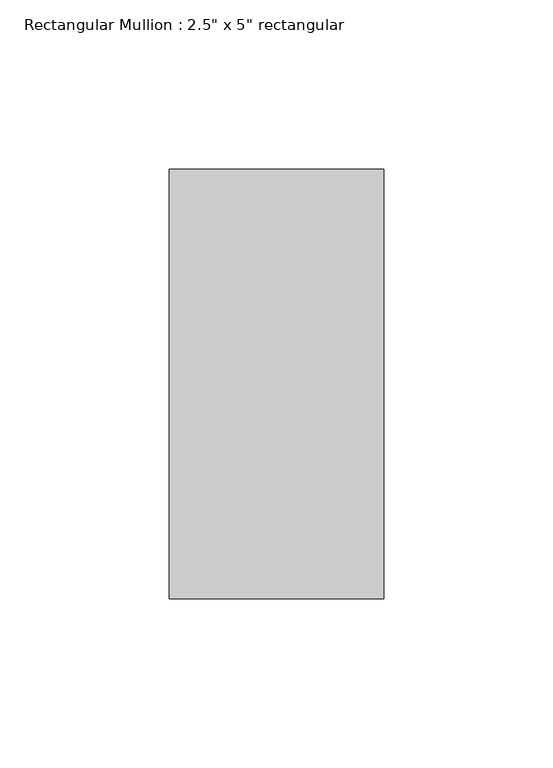
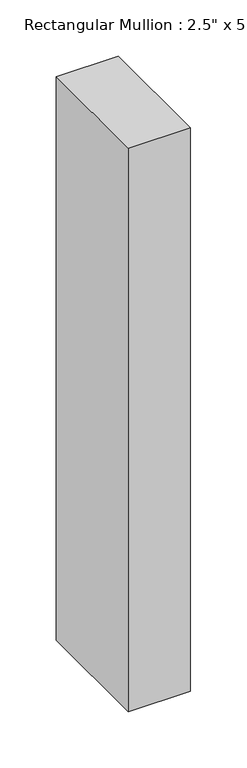
"""IFC4 building model written with IfcOpenShell, lengths in millimetres: member geometry."""

from ifc_helpers import new_model, si_unit, frame, origin, place, context, project, spatial, polyline, outline, extrude, source, transform, mapped, element, save


def member_6e77e263(model_context):
    return source(origin(), model_context, "Body", "SweptSolid", [
        extrude(outline(polyline([(31.75, 63.5), (31.75, -63.5), (-31.75, -63.5), (-31.75, 63.5), (31.75, 63.5)])), frame((0.0, 0.0, -609.6), z_axis=(0.0, 0.0, 1.0), x_axis=(1.0, 0.0, 0.0)), (0.0, 0.0, 1.0), 609.6),
    ])


if __name__ == "__main__":
    model = new_model("IFC4")
    model_context = context("Model", 3, world=origin())
    ifc_project = project(units=[si_unit("LENGTHUNIT", "METRE", prefix="MILLI")], contexts=[model_context])
    site = spatial("IfcSite", under=ifc_project)
    building = spatial("IfcBuilding", under=site)
    placement = place(None, origin())
    member_shape = member_6e77e263(model_context)
    element("IfcMember", 1, ObjectType="Rectangular Mullion : 2.5\" x 5\" rectangular", at=placement, inside=building, context=model_context, shape_type="MappedRepresentation", body=[
        mapped(member_shape, transform((0.0, 0.0, 0.0), x_axis=(1.0, 0.0, 0.0), y_axis=(0.0, 1.0, 0.0), z_axis=(0.0, 0.0, 1.0))),
    ])
    save(model, "model.ifc")

# Revit data of these elements
# Type "Rectangular Mullion : 2.5\" x 5\" rectangular"
#   built-in parameter 1007304 = 0.416667 (stored number, unit not read)
#   built-in parameter 1007301 = 0.104167 (stored number, unit not read)
#   built-in parameter 1007300 = 0.104167 (stored number, unit not read)
# Element 1 (IfcMember, "Rectangular Mullion : 2.5\" x 5\" rectangular")
#   Materials on its faces: "Aluminum"
# Materials
#   "Aluminum": class "Metal", colour RGB 247 247 247, transparency 0, Description = "Aluminum 6061", Cost = 0
